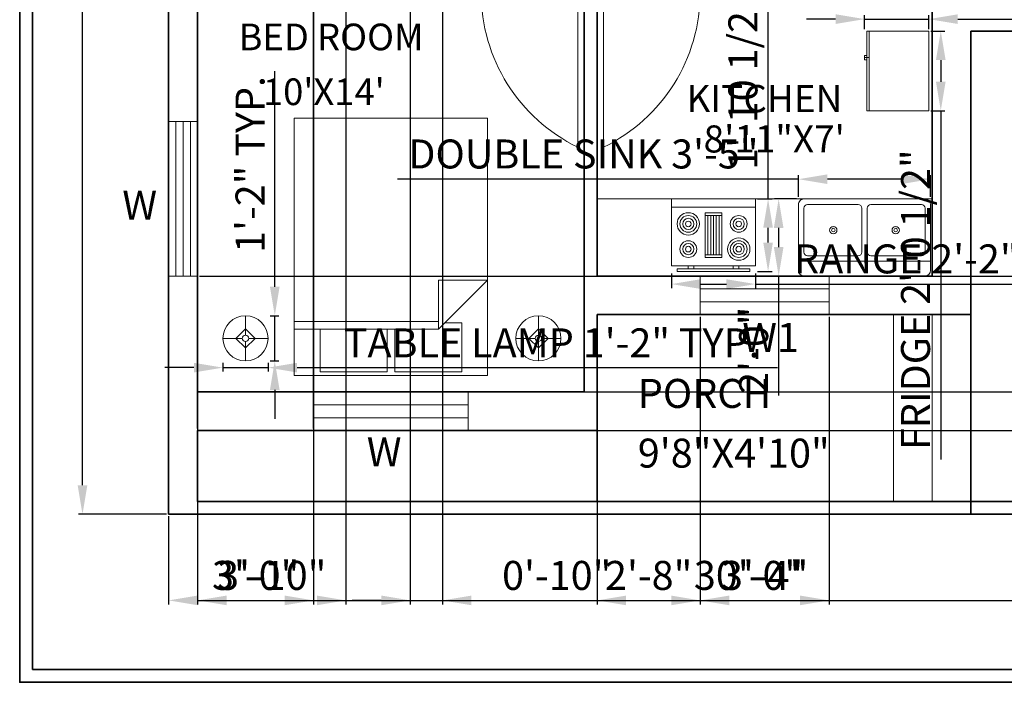
# Model space of a CAD drawing. Units: inches. Extents: x 2436 to 3928, y 1526 to 2149.
# Tile 1 of 6: x 2436 to 2742, y 1526 to 1731. Entities that reach past the tile are written whole.
import ezdxf

# ---------------------------------------------------------------- set-up
doc = ezdxf.new("R2010")
doc.units = ezdxf.units.IN
for name, color, linetype, lineweight in [('A-AREA-IDEN', 152, 'Continuous', 18), ('A-DOOR', 4, 'Continuous', 18), ('A-EQPM', 9, 'Continuous', 18), ('A-FLOR-CASE', 8, 'Continuous', 18), ('A-FLOR-FIXT', 9, 'Continuous', 18), ('A-FLOR-STRS', 7, 'Continuous', 18), ('A-FURN', 8, 'Continuous', 18), ('A-GLAZ', 2, 'Continuous', 18), ('A-GLAZ-TEXT', 114, 'Continuous', 18), ('A-WALL', 7, 'Continuous', 35), ('G-ANNO-TTLB', 7, 'Continuous', 35), ('S-ANNO-DIMS', 2, 'Continuous', 18)]:
    doc.layers.add(name, color=color, linetype=linetype, lineweight=lineweight)
doc.styles.get("Standard").update_dxf_attribs({"font": 'arial.ttf'})
doc.dimstyles.new('ISO-25', dxfattribs={"dimtxt": 9, "dimasz": 9, "dimexe": 1.25, "dimexo": 0.625, "dimgap": 2, "dimtad": 1, "dimdec": 1, "dimlunit": 4, "dimtxsty": 'Standard', "dimcen": 2.5, "dimadec": 0, "dimazin": 0, "dimtfac": 1, "dimtdec": 1, "dimtmove": 0, "dimatfit": 3, "dimfxl": 1, "dimarcsym": 0})

# ---------------------------------------------------------------- blocks, each defined once
blk = doc.blocks.new('Range-Oven - 30 in top')
for p, q in [((0, -3), (30, -3)), ((12, -6), (18, -6)), ((13, -20), (13, -6)), ((14, -6), (14, -20)), ((15, -20), (15, -6)), ((16, -6), (16, -20)), ((17, -20), (17, -6)), ((18, -20), (12, -20)), ((6, -24), (6, -25)), ((8, -25), (8, -24)), ((22, -25), (22, -24)), ((24, -24), (24, -25))]:
    blk.add_line(p, q)
for points in [[(0, -24), (0, 0), (30, 0), (30, -24)], [(12, -21), (12, -5), (18, -5), (18, -21)], [(2, -26), (2, -25), (28, -25), (28, -26)]]:
    blk.add_lwpolyline(points, close=True)
for centre, radius in [((6, -9), 4), ((6, -9), 3), ((6, -9), 2), ((24, -9), 3), ((24, -9), 2), ((6, -9), 1), ((24, -9), 1), ((24, -18), 4), ((6, -18), 3), ((6, -18), 2), ((6, -18), 1), ((24, -18), 3), ((24, -18), 2), ((24, -18), 1)]:
    blk.add_circle(centre, radius)
blk = doc.blocks.new('Sink-double - 36 in top')
for p, q in [((-18, -4), (18, -4)), ((-0.75, -18.5), (-0.75, -6.5)), ((0.75, -6.5), (0.75, -18.5))]:
    blk.add_line(p, q)
for points in [[(-16.5, 0), (16.5, 0)], [(-18, -19.5), (-18, -1.5)], [(18, -1.5), (18, -19.5)], [(-16.5, -18.5), (-16.5, -6.5)], [(-15.5, -5.5), (-1.75, -5.5)], [(1.75, -5.5), (15.5, -5.5)], [(16.5, -6.5), (16.5, -18.5)], [(16.5, -21), (-16.5, -21)], [(-1.75, -19.5), (-15.5, -19.5)], [(15.5, -19.5), (1.75, -19.5)]]:
    blk.add_lwpolyline(points)
for centre, radius in [((-8.5, -12.5), 1), ((-8.5, -12.5), 0.5), ((8.5, -12.5), 1), ((8.5, -12.5), 0.5)]:
    blk.add_circle(centre, radius)
for centre, radius, start, end in [((-16.5, -1.5), 1.5, 90, 180), ((16.5, -1.5), 1.5, 0, 90), ((-15.5, -6.5), 1, 90, 180), ((-1.75, -6.5), 1, 0, 90), ((1.75, -6.5), 1, 90, 180), ((15.5, -6.5), 1, 0, 90), ((-15.5, -18.5), 1, 180, 270), ((-1.75, -18.5), 1, 270, 0), ((1.75, -18.5), 1, 180, 270), ((15.5, -18.5), 1, 270, 0), ((-16.5, -19.5), 1.5, 180, 270), ((16.5, -19.5), 1.5, 270, 0)]:
    blk.add_arc(centre, radius, start, end)
blk = doc.blocks.new('Refrigerator-2 door - 36 in top')
for p, q in [((0, -26.999999), (36, -26.999999)), ((11, -27.999999), (11, -28.999999)), ((11, -28.999999), (13, -28.999999)), ((12, -26.999999), (12, -28.999999)), ((13, -28.999999), (13, -27.999999))]:
    blk.add_line(p, q)
blk.add_lwpolyline([(0, -27.999999), (0, 0), (36, 0), (36, -27.999999)], close=True)
blk = doc.blocks.new('Bed - Queen')
for p, q in [((0, -80.00003), (0, 0)), ((0, 0), (59.99999, 0)), ((59.99999, 0), (59.99999, -80.00003)), ((7.99999, -1.2), (28.79998, -1.2)), ((7.99999, -14.4), (7.99999, -1.2)), ((28.79998, -1.2), (28.79998, -14.4)), ((31.19999, -1.2), (51.99999, -1.2)), ((31.19999, -14.4), (31.19999, -1.2)), ((51.99999, -1.2), (51.99999, -16.4)), ((0, -14.4), (44.8, -14.4)), ((59.99999, -29.6), (44.8, -14.4)), ((44.8, -14.4), (44.8, -29.6)), ((44.8, -16.8), (0, -16.8)), ((51.99999, -16.4), (46.79936, -16.4)), ((44.8, -29.6), (59.99999, -29.6)), ((59.99999, -80.00003), (0, -80.00003))]:
    blk.add_line(p, q)
blk = doc.blocks.new('Lamp - Table')
for p, q in [((0, 7), (0, 1)), ((-1, 0), (-7, 0)), ((0, 3), (-3, 0)), ((-3, 0), (0, -3)), ((3, 0), (0, 3)), ((0, -3), (3, 0)), ((1, 0), (7, 0)), ((0, -1), (0, -7))]:
    blk.add_line(p, q)
for radius in [7, 1]:
    blk.add_circle((0, 0), radius)
blk = doc.blocks.new('WIN-48x9-PLAN')
for p, q in [((0, 0), (0, 9)), ((0, 6.75), (48, 6.75)), ((48, 0), (48, 9)), ((0, 4.5), (48, 4.5)), ((0, 2.25), (48, 2.25))]:
    blk.add_line(p, q)
blk = doc.blocks.new('DOOR-SINGLE-30-PLAN')
blk.add_line((0, 0), (0, 48))
blk.add_arc((-23.4, 0), 53.4, 0, 64.0108)
blk = doc.blocks.new('*D32')
at = {"layer": 'Defpoints', "color": 0, "transparency": 16777216}
for p in [(2499.08, 1625.43), (2513.08, 1625.43), (2513.08, 1623.33)]:
    blk.add_point(p, dxfattribs=at)
at = {"layer": 'S-ANNO-DIMS', "color": 0, "lineweight": -2, "transparency": 16777216}
for p, q in [((2490.08, 1623.33), (2481.08, 1623.33)), ((2499.08, 1624.8), (2499.08, 1622.08)), ((2499.08, 1623.33), (2513.08, 1623.33)), ((2513.08, 1624.8), (2513.08, 1622.08)), ((2522.08, 1623.33), (2671.22, 1623.33))]:
    blk.add_line(p, q, dxfattribs=at)
at = {"layer": 'S-ANNO-DIMS', "color": 0, "transparency": 16777216}
for points in [[(2490.08, 1624.83), (2490.08, 1621.83), (2499.08, 1623.33)], [(2522.08, 1624.83), (2522.08, 1621.83), (2513.08, 1623.33)]]:
    blk.add_solid(points, dxfattribs=at)
at = {"layer": 'S-ANNO-DIMS', "color": 0, "transparency": 16777216, "insert": (2601.15, 1629.85), "char_height": 9, "attachment_point": 5}
blk.add_mtext('TABLE LAMP 1\'-2" TYP.', dxfattribs=at)
blk = doc.blocks.new('*D33')
at = {"layer": 'Defpoints', "color": 0, "transparency": 16777216}
for p in [(2513.08, 1639.43), (2515.18, 1639.43), (2513.08, 1625.43)]:
    blk.add_point(p, dxfattribs=at)
at = {"layer": 'S-ANNO-DIMS', "color": 0, "lineweight": -2, "transparency": 16777216}
for p, q in [((2515.18, 1648.43), (2515.18, 1715.44)), ((2513.7, 1639.43), (2516.43, 1639.43)), ((2515.18, 1625.43), (2515.18, 1639.43)), ((2513.7, 1625.43), (2516.43, 1625.43)), ((2515.18, 1616.43), (2515.18, 1607.43))]:
    blk.add_line(p, q, dxfattribs=at)
at = {"layer": 'S-ANNO-DIMS', "color": 0, "transparency": 16777216}
for points in [[(2513.68, 1648.43), (2516.68, 1648.43), (2515.18, 1639.43)], [(2513.68, 1616.43), (2516.68, 1616.43), (2515.18, 1625.43)]]:
    blk.add_solid(points, dxfattribs=at)
at = {"layer": 'S-ANNO-DIMS', "color": 0, "transparency": 16777216, "insert": (2508.66, 1686.43), "char_height": 9, "attachment_point": 5, "rotation": 90}
blk.add_mtext('1\'-2" TYP.', dxfattribs=at)
blk = doc.blocks.new('*D50')
at = {"layer": 'Defpoints', "color": 0, "transparency": 16777216}
for p in [(2638.33, 1653.19), (2664.4, 1653.19), (2664.4, 1649.28)]:
    blk.add_point(p, dxfattribs=at)
at = {"layer": 'S-ANNO-DIMS', "color": 0, "lineweight": -2, "transparency": 16777216}
for p, q in [((2638.33, 1652.56), (2638.33, 1648.03)), ((2664.4, 1652.56), (2664.4, 1648.03)), ((2647.33, 1649.28), (2655.4, 1649.28)), ((2664.4, 1649.28), (2749.06, 1649.28))]:
    blk.add_line(p, q, dxfattribs=at)
at = {"layer": 'S-ANNO-DIMS', "color": 0, "transparency": 16777216}
for points in [[(2647.33, 1650.78), (2647.33, 1647.78), (2638.33, 1649.28)], [(2655.4, 1650.78), (2655.4, 1647.78), (2664.4, 1649.28)]]:
    blk.add_solid(points, dxfattribs=at)
at = {"layer": 'S-ANNO-DIMS', "color": 0, "transparency": 16777216, "insert": (2711.23, 1655.93), "char_height": 9, "attachment_point": 5}
blk.add_mtext('RANGE 2\'-2"', dxfattribs=at)
blk = doc.blocks.new('*D51')
at = {"layer": 'Defpoints', "color": 0, "transparency": 16777216}
for p in [(2664.4, 1675.79), (2668.31, 1675.79), (2664.4, 1653.19)]:
    blk.add_point(p, dxfattribs=at)
at = {"layer": 'S-ANNO-DIMS', "color": 0, "lineweight": -2, "transparency": 16777216}
for p, q in [((2668.31, 1675.79), (2668.31, 1739.83)), ((2665.03, 1675.79), (2669.56, 1675.79)), ((2668.31, 1662.19), (2668.31, 1666.79)), ((2665.03, 1653.19), (2669.56, 1653.19))]:
    blk.add_line(p, q, dxfattribs=at)
at = {"layer": 'S-ANNO-DIMS', "color": 0, "transparency": 16777216}
for points in [[(2666.81, 1666.79), (2669.81, 1666.79), (2668.31, 1675.79)], [(2666.81, 1662.19), (2669.81, 1662.19), (2668.31, 1653.19)]]:
    blk.add_solid(points, dxfattribs=at)
at = {"layer": 'S-ANNO-DIMS', "color": 0, "transparency": 16777216, "insert": (2661.66, 1712.31), "char_height": 9, "attachment_point": 5, "rotation": 90}
blk.add_mtext('1\'-10 1/2"', dxfattribs=at)
blk = doc.blocks.new('*D52')
at = {"layer": 'Defpoints', "color": 0, "transparency": 16777216}
for p in [(2677.74, 1681.86), (2677.74, 1675.71), (2718.75, 1675.71)]:
    blk.add_point(p, dxfattribs=at)
at = {"layer": 'S-ANNO-DIMS', "color": 0, "lineweight": -2, "transparency": 16777216}
for p, q in [((2677.74, 1681.86), (2553.23, 1681.86)), ((2677.74, 1676.34), (2677.74, 1683.11)), ((2709.75, 1681.86), (2686.74, 1681.86)), ((2718.75, 1676.34), (2718.75, 1683.11))]:
    blk.add_line(p, q, dxfattribs=at)
at = {"layer": 'S-ANNO-DIMS', "color": 0, "transparency": 16777216}
for points in [[(2686.74, 1683.36), (2686.74, 1680.36), (2677.74, 1681.86)], [(2709.75, 1683.36), (2709.75, 1680.36), (2718.75, 1681.86)]]:
    blk.add_solid(points, dxfattribs=at)
at = {"layer": 'S-ANNO-DIMS', "color": 0, "transparency": 16777216, "insert": (2610.98, 1688.52), "char_height": 9, "attachment_point": 5}
blk.add_mtext('DOUBLE SINK 3\'-5"', dxfattribs=at)
blk = doc.blocks.new('*D53')
at = {"layer": 'Defpoints', "color": 0, "transparency": 16777216}
for p in [(2677.74, 1675.71), (2671.59, 1651.79), (2677.74, 1651.79)]:
    blk.add_point(p, dxfattribs=at)
at = {"layer": 'S-ANNO-DIMS', "color": 0, "lineweight": -2, "transparency": 16777216}
for p, q in [((2677.11, 1675.71), (2670.34, 1675.71)), ((2671.59, 1666.71), (2671.59, 1660.79)), ((2677.11, 1651.79), (2670.34, 1651.79)), ((2671.59, 1651.79), (2671.59, 1614.71))]:
    blk.add_line(p, q, dxfattribs=at)
at = {"layer": 'S-ANNO-DIMS', "color": 0, "transparency": 16777216}
for points in [[(2670.09, 1666.71), (2673.09, 1666.71), (2671.59, 1675.71)], [(2670.09, 1660.79), (2673.09, 1660.79), (2671.59, 1651.79)]]:
    blk.add_solid(points, dxfattribs=at)
at = {"layer": 'S-ANNO-DIMS', "color": 0, "transparency": 16777216, "insert": (2664.99, 1628.75), "char_height": 9, "attachment_point": 5, "rotation": 90}
blk.add_mtext('2\'-0"', dxfattribs=at)
blk = doc.blocks.new('*D54')
at = {"layer": 'Defpoints', "color": 0, "transparency": 16777216}
for p in [(2718.2, 1727.86), (2718.2, 1703.12), (2721.91, 1703.12)]:
    blk.add_point(p, dxfattribs=at)
at = {"layer": 'S-ANNO-DIMS', "color": 0, "lineweight": -2, "transparency": 16777216}
for p, q in [((2718.82, 1727.86), (2723.16, 1727.86)), ((2721.91, 1718.86), (2721.91, 1712.12)), ((2718.82, 1703.12), (2723.16, 1703.12)), ((2721.91, 1703.12), (2721.91, 1594.75))]:
    blk.add_line(p, q, dxfattribs=at)
at = {"layer": 'S-ANNO-DIMS', "color": 0, "transparency": 16777216}
for points in [[(2720.41, 1718.86), (2723.41, 1718.86), (2721.91, 1727.86)], [(2720.41, 1712.12), (2723.41, 1712.12), (2721.91, 1703.12)]]:
    blk.add_solid(points, dxfattribs=at)
at = {"layer": 'S-ANNO-DIMS', "color": 0, "transparency": 16777216, "insert": (2715.25, 1644.44), "char_height": 9, "attachment_point": 5, "rotation": 90}
blk.add_mtext('FRIDGE 2\'-0 1/2"', dxfattribs=at)
blk = doc.blocks.new('*D55')
at = {"layer": 'Defpoints', "color": 0, "transparency": 16777216}
for p in [(2718.2, 1731.57), (2698.27, 1727.86), (2718.2, 1727.86)]:
    blk.add_point(p, dxfattribs=at)
at = {"layer": 'S-ANNO-DIMS', "color": 0, "lineweight": -2, "transparency": 16777216}
for p, q in [((2689.27, 1731.57), (2680.27, 1731.57)), ((2698.27, 1728.48), (2698.27, 1732.82)), ((2698.27, 1731.57), (2718.2, 1731.57)), ((2718.2, 1728.48), (2718.2, 1732.82)), ((2727.2, 1731.57), (2763.27, 1731.57))]:
    blk.add_line(p, q, dxfattribs=at)
at = {"layer": 'S-ANNO-DIMS', "color": 0, "transparency": 16777216}
for points in [[(2689.27, 1733.07), (2689.27, 1730.07), (2698.27, 1731.57)], [(2727.2, 1733.07), (2727.2, 1730.07), (2718.2, 1731.57)]]:
    blk.add_solid(points, dxfattribs=at)
at = {"layer": 'S-ANNO-DIMS', "color": 0, "transparency": 16777216, "insert": (2749.73, 1738.16), "char_height": 9, "attachment_point": 5}
blk.add_mtext('1\'-8"', dxfattribs=at)
blk = doc.blocks.new('*D56')
at = {"layer": 'Defpoints', "color": 0, "transparency": 16777216}
for p in [(2482.24, 1577.79), (2842.24, 1577.79), (2842.24, 1551.04)]:
    blk.add_point(p, dxfattribs=at)
at = {"layer": 'S-ANNO-DIMS', "color": 0, "lineweight": -2, "transparency": 16777216}
for p, q in [((2482.24, 1577.16), (2482.24, 1549.79)), ((2842.24, 1577.16), (2842.24, 1549.79)), ((2491.24, 1551.04), (2833.24, 1551.04))]:
    blk.add_line(p, q, dxfattribs=at)
at = {"layer": 'S-ANNO-DIMS', "color": 0, "transparency": 16777216}
for points in [[(2491.24, 1552.54), (2491.24, 1549.54), (2482.24, 1551.04)], [(2833.24, 1552.54), (2833.24, 1549.54), (2842.24, 1551.04)]]:
    blk.add_solid(points, dxfattribs=at)
at = {"layer": 'S-ANNO-DIMS', "color": 0, "transparency": 16777216, "insert": (2662.24, 1557.64), "char_height": 9, "attachment_point": 5}
blk.add_mtext('30\'-0"', dxfattribs=at)
blk = doc.blocks.new('*D57')
at = {"layer": 'Defpoints', "color": 0, "transparency": 16777216}
for p in [(2455.49, 2017.79), (2482.24, 2017.79), (2482.24, 1577.79)]:
    blk.add_point(p, dxfattribs=at)
at = {"layer": 'S-ANNO-DIMS', "color": 0, "lineweight": -2, "transparency": 16777216}
for p, q in [((2481.61, 2017.79), (2454.24, 2017.79)), ((2455.49, 1586.79), (2455.49, 2008.79)), ((2481.61, 1577.79), (2454.24, 1577.79))]:
    blk.add_line(p, q, dxfattribs=at)
at = {"layer": 'S-ANNO-DIMS', "color": 0, "transparency": 16777216}
for points in [[(2453.99, 2008.79), (2456.99, 2008.79), (2455.49, 2017.79)], [(2453.99, 1586.79), (2456.99, 1586.79), (2455.49, 1577.79)]]:
    blk.add_solid(points, dxfattribs=at)
at = {"layer": 'S-ANNO-DIMS', "color": 0, "transparency": 16777216, "insert": (2448.89, 1797.79), "char_height": 9, "attachment_point": 5, "rotation": 90}
blk.add_mtext('36\'-8"', dxfattribs=at)
blk = doc.blocks.new('*D58')
at = {"layer": 'Defpoints', "color": 0, "transparency": 16777216}
for p in [(2491.24, 2008.79), (2527.24, 2008.79), (2527.24, 1551.04)]:
    blk.add_point(p, dxfattribs=at)
at = {"layer": 'S-ANNO-DIMS', "color": 0, "lineweight": -2, "transparency": 16777216}
for p, q in [((2491.24, 2008.16), (2491.24, 1549.79)), ((2527.24, 2008.16), (2527.24, 1549.79)), ((2500.24, 1551.04), (2518.24, 1551.04))]:
    blk.add_line(p, q, dxfattribs=at)
at = {"layer": 'S-ANNO-DIMS', "color": 0, "transparency": 16777216}
for points in [[(2500.24, 1552.54), (2500.24, 1549.54), (2491.24, 1551.04)], [(2518.24, 1552.54), (2518.24, 1549.54), (2527.24, 1551.04)]]:
    blk.add_solid(points, dxfattribs=at)
at = {"layer": 'S-ANNO-DIMS', "color": 0, "transparency": 16777216, "insert": (2509.24, 1557.64), "char_height": 9, "attachment_point": 5}
blk.add_mtext('3\'-0"', dxfattribs=at)
blk = doc.blocks.new('*D63')
at = {"layer": 'Defpoints', "color": 0, "transparency": 16777216}
for p in [(2491.24, 1651.79), (2868.99, 1651.79), (2491.24, 1615.79)]:
    blk.add_point(p, dxfattribs=at)
at = {"layer": 'S-ANNO-DIMS', "color": 0, "lineweight": -2, "transparency": 16777216}
for p, q in [((2491.86, 1651.79), (2870.24, 1651.79)), ((2868.99, 1624.79), (2868.99, 1642.79)), ((2491.86, 1615.79), (2870.24, 1615.79))]:
    blk.add_line(p, q, dxfattribs=at)
at = {"layer": 'S-ANNO-DIMS', "color": 0, "transparency": 16777216}
for points in [[(2867.49, 1642.79), (2870.49, 1642.79), (2868.99, 1651.79)], [(2867.49, 1624.79), (2870.49, 1624.79), (2868.99, 1615.79)]]:
    blk.add_solid(points, dxfattribs=at)
at = {"layer": 'S-ANNO-DIMS', "color": 0, "transparency": 16777216, "insert": (2862.39, 1633.79), "char_height": 9, "attachment_point": 5, "rotation": 90}
blk.add_mtext('3\'-0"', dxfattribs=at)
blk = doc.blocks.new('*D64')
at = {"layer": 'Defpoints', "color": 0, "transparency": 16777216}
for p in [(2527.24, 2114.67), (2491.24, 1603.79), (2527.24, 1603.79)]:
    blk.add_point(p, dxfattribs=at)
at = {"layer": 'S-ANNO-DIMS', "color": 0, "lineweight": -2, "transparency": 16777216}
for p, q in [((2491.24, 1604.41), (2491.24, 2115.92)), ((2527.24, 1604.41), (2527.24, 2115.92)), ((2500.24, 2114.67), (2518.24, 2114.67))]:
    blk.add_line(p, q, dxfattribs=at)
at = {"layer": 'S-ANNO-DIMS', "color": 0, "transparency": 16777216}
for points in [[(2500.24, 2116.17), (2500.24, 2113.17), (2491.24, 2114.67)], [(2518.24, 2116.17), (2518.24, 2113.17), (2527.24, 2114.67)]]:
    blk.add_solid(points, dxfattribs=at)
at = {"layer": 'S-ANNO-DIMS', "color": 0, "transparency": 16777216, "insert": (2509.24, 2121.27), "char_height": 9, "attachment_point": 5}
blk.add_mtext('3\'-0"', dxfattribs=at)
blk = doc.blocks.new('*D65')
at = {"layer": 'Defpoints', "color": 0, "transparency": 16777216}
for p in [(2575.24, 1615.79), (2868.99, 1615.79), (2575.24, 1603.79)]:
    blk.add_point(p, dxfattribs=at)
at = {"layer": 'S-ANNO-DIMS', "color": 0, "lineweight": -2, "transparency": 16777216}
for p, q in [((2868.99, 1624.79), (2868.99, 1660.87)), ((2575.86, 1615.79), (2870.24, 1615.79)), ((2868.99, 1603.79), (2868.99, 1615.79)), ((2575.86, 1603.79), (2870.24, 1603.79)), ((2868.99, 1594.79), (2868.99, 1585.79))]:
    blk.add_line(p, q, dxfattribs=at)
at = {"layer": 'S-ANNO-DIMS', "color": 0, "transparency": 16777216}
for points in [[(2867.49, 1624.79), (2870.49, 1624.79), (2868.99, 1615.79)], [(2867.49, 1594.79), (2870.49, 1594.79), (2868.99, 1603.79)]]:
    blk.add_solid(points, dxfattribs=at)
at = {"layer": 'S-ANNO-DIMS', "color": 0, "transparency": 16777216, "insert": (2862.39, 1647.33), "char_height": 9, "attachment_point": 5, "rotation": 90}
blk.add_mtext('1\'-0"', dxfattribs=at)
blk = doc.blocks.new('*D66')
at = {"layer": 'Defpoints', "color": 0, "transparency": 16777216}
for p in [(2647.24, 1639.79), (2687.24, 1639.79), (2687.24, 1551.04)]:
    blk.add_point(p, dxfattribs=at)
at = {"layer": 'S-ANNO-DIMS', "color": 0, "lineweight": -2, "transparency": 16777216}
for p, q in [((2647.24, 1639.16), (2647.24, 1549.79)), ((2687.24, 1639.16), (2687.24, 1549.79)), ((2656.24, 1551.04), (2678.24, 1551.04))]:
    blk.add_line(p, q, dxfattribs=at)
at = {"layer": 'S-ANNO-DIMS', "color": 0, "transparency": 16777216}
for points in [[(2656.24, 1552.54), (2656.24, 1549.54), (2647.24, 1551.04)], [(2678.24, 1552.54), (2678.24, 1549.54), (2687.24, 1551.04)]]:
    blk.add_solid(points, dxfattribs=at)
at = {"layer": 'S-ANNO-DIMS', "color": 0, "transparency": 16777216, "insert": (2667.24, 1557.64), "char_height": 9, "attachment_point": 5}
blk.add_mtext('3\'-4"', dxfattribs=at)
blk = doc.blocks.new('*D67')
at = {"layer": 'Defpoints', "color": 0, "transparency": 16777216}
for p in [(2615.24, 1639.79), (2647.24, 1639.79), (2647.24, 1551.04)]:
    blk.add_point(p, dxfattribs=at)
at = {"layer": 'S-ANNO-DIMS', "color": 0, "lineweight": -2, "transparency": 16777216}
for p, q in [((2615.24, 1639.16), (2615.24, 1549.79)), ((2647.24, 1639.16), (2647.24, 1549.79)), ((2624.24, 1551.04), (2638.24, 1551.04))]:
    blk.add_line(p, q, dxfattribs=at)
at = {"layer": 'S-ANNO-DIMS', "color": 0, "transparency": 16777216}
for points in [[(2624.24, 1552.54), (2624.24, 1549.54), (2615.24, 1551.04)], [(2638.24, 1552.54), (2638.24, 1549.54), (2647.24, 1551.04)]]:
    blk.add_solid(points, dxfattribs=at)
at = {"layer": 'S-ANNO-DIMS', "color": 0, "transparency": 16777216, "insert": (2631.24, 1557.63), "char_height": 9, "attachment_point": 5}
blk.add_mtext('2\'-8"', dxfattribs=at)
blk = doc.blocks.new('*D72')
at = {"layer": 'Defpoints', "color": 0, "transparency": 16777216}
for p in [(2491.24, 1798.29), (2537.24, 1788.29), (2537.24, 1551.04)]:
    blk.add_point(p, dxfattribs=at)
at = {"layer": 'S-ANNO-DIMS', "color": 0, "lineweight": -2, "transparency": 16777216}
for p, q in [((2491.24, 1797.66), (2491.24, 1549.79)), ((2537.24, 1787.66), (2537.24, 1549.79)), ((2500.24, 1551.04), (2528.24, 1551.04))]:
    blk.add_line(p, q, dxfattribs=at)
at = {"layer": 'S-ANNO-DIMS', "color": 0, "transparency": 16777216}
for points in [[(2500.24, 1552.54), (2500.24, 1549.54), (2491.24, 1551.04)], [(2528.24, 1552.54), (2528.24, 1549.54), (2537.24, 1551.04)]]:
    blk.add_solid(points, dxfattribs=at)
at = {"layer": 'S-ANNO-DIMS', "color": 0, "transparency": 16777216, "insert": (2514.24, 1557.64), "char_height": 9, "attachment_point": 5}
blk.add_mtext('3\'-10"', dxfattribs=at)
blk = doc.blocks.new('*D73')
at = {"layer": 'Defpoints', "color": 0, "transparency": 16777216}
for p in [(2557.24, 1798.29), (2567.24, 1798.29), (2567.24, 1551.04)]:
    blk.add_point(p, dxfattribs=at)
at = {"layer": 'S-ANNO-DIMS', "color": 0, "lineweight": -2, "transparency": 16777216}
for p, q in [((2557.24, 1797.66), (2557.24, 1549.79)), ((2567.24, 1797.66), (2567.24, 1549.79)), ((2548.24, 1551.04), (2539.24, 1551.04)), ((2557.24, 1551.04), (2567.24, 1551.04)), ((2576.24, 1551.04), (2620.16, 1551.04))]:
    blk.add_line(p, q, dxfattribs=at)
at = {"layer": 'S-ANNO-DIMS', "color": 0, "transparency": 16777216}
for points in [[(2548.24, 1552.54), (2548.24, 1549.54), (2557.24, 1551.04)], [(2576.24, 1552.54), (2576.24, 1549.54), (2567.24, 1551.04)]]:
    blk.add_solid(points, dxfattribs=at)
at = {"layer": 'S-ANNO-DIMS', "color": 0, "transparency": 16777216, "insert": (2602.7, 1557.63), "char_height": 9, "attachment_point": 5}
blk.add_mtext('0\'-10"', dxfattribs=at)

msp = doc.modelspace()

# ---------------------------------------------------------------- linework, layer by layer
at = {"layer": 'A-FLOR-CASE'}
msp.add_line((2615.24, 1675.79), (2719.24, 1675.79), dxfattribs=at)
at = {"layer": 'A-FLOR-STRS'}
for p, q in [((2707.24, 1581.79), (2707.24, 1639.79)), ((2719.24, 1581.79), (2719.24, 1639.79))]:
    msp.add_line(p, q, dxfattribs=at)
at = {"layer": 'A-GLAZ'}
for p, q in [((2647.24, 1651.79), (2647.24, 1639.79)), ((2687.24, 1651.79), (2687.24, 1639.79)), ((2647.24, 1647.79), (2687.24, 1647.79)), ((2647.24, 1643.79), (2687.24, 1643.79)), ((2527.24, 1615.79), (2527.24, 1603.79)), ((2575.24, 1615.79), (2575.24, 1603.79)), ((2527.24, 1611.79), (2575.24, 1611.79)), ((2527.24, 1607.79), (2575.24, 1607.79))]:
    msp.add_line(p, q, dxfattribs=at)
at = {"layer": 'A-WALL'}
for p, q in [((2482.24, 1577.79), (2482.24, 2017.79)), ((2491.24, 1615.79), (2491.24, 1735.79)), ((2611.24, 1615.79), (2611.24, 1735.79)), ((2615.24, 1651.79), (2615.24, 1735.79)), ((2719.24, 1651.79), (2719.24, 1735.79)), ((2731.24, 1577.79), (2731.24, 1727.79)), ((2731.24, 1727.79), (2783.24, 1727.79)), ((2615.24, 1651.79), (2719.24, 1651.79)), ((2615.24, 1581.79), (2615.24, 1639.79)), ((2615.24, 1639.79), (2731.24, 1639.79)), ((2491.24, 1615.79), (2611.24, 1615.79)), ((2482.24, 1577.79), (2482.24, 1603.79)), ((2491.24, 1581.79), (2491.24, 1603.79)), ((2491.24, 1603.79), (2615.24, 1603.79)), ((2482.24, 1581.79), (2482.24, 1595.79)), ((2491.24, 1581.79), (2833.24, 1581.79)), ((2482.24, 1577.79), (2842.24, 1577.79))]:
    msp.add_line(p, q, dxfattribs=at)
at = {"layer": 'G-ANNO-TTLB'}
for points in [[(2436, 2138.4), (3927.51, 2138.4), (3927.51, 1525.6), (2436, 1525.6)], [(2440, 2134.4), (3923.51, 2134.4), (3923.51, 1529.6), (2440, 1529.6)]]:
    msp.add_lwpolyline(points, close=True, dxfattribs=at)

# ---------------------------------------------------------------- block references
at = {"layer": 'A-DOOR', "rotation": 180}
msp.add_blockref('DOOR-SINGLE-30-PLAN', (2609.24, 1739.79), dxfattribs=at)
at = {"layer": 'A-DOOR', "extrusion": (0, 0, -1), "zscale": -1, "rotation": 180}
msp.add_blockref('DOOR-SINGLE-30-PLAN', (-2617.24, 1739.79), dxfattribs=at)
at = {"layer": 'A-EQPM', "xscale": 0.6870046739389232, "yscale": 0.6870046739389232, "zscale": 0.6870046739389232, "rotation": 270}
msp.add_blockref('Refrigerator-2 door - 36 in top', (2718.2, 1727.86), dxfattribs=at)
at = {"layer": 'A-EQPM', "xscale": 0.8692268544197554, "yscale": 0.8692268544197554, "zscale": 0.8692268544197554}
msp.add_blockref('Range-Oven - 30 in top', (2638.33, 1675.79), dxfattribs=at)
at = {"layer": 'A-FLOR-FIXT', "xscale": 1.139099176884385, "yscale": 1.139099176884385, "zscale": 1.139099176884385, "rotation": 180}
msp.add_blockref('Sink-double - 36 in top', (2698.24, 1651.79), dxfattribs=at)
at = {"layer": 'A-FURN', "xscale": -1, "rotation": 180}
msp.add_blockref('Bed - Queen', (2521.24, 1620.85), dxfattribs=at)
at = {"layer": 'A-FURN'}
for p in [(2506.08, 1632.43), (2597.01, 1632.43)]:
    msp.add_blockref('Lamp - Table', p, dxfattribs=at)
at = {"layer": 'A-GLAZ', "rotation": 270.0000000000031}
msp.add_blockref('WIN-48x9-PLAN', (2482.24, 1699.79), dxfattribs=at)

# ---------------------------------------------------------------- texts
at = {"layer": 'A-AREA-IDEN'}
for s, height, p in [('BED ROOM', 8.272, (2503.94, 1721.9)), ("   10'X14'", 8.272, (2503.94, 1704.87)), ('KITCHEN', 8.409, (2642.97, 1702.68)), ('8\'11"X7\'', 8.409, (2648.29, 1690.16)), ('PORCH', 9, (2627.87, 1610.82)), ('9\'8"X4\'10"', 9, (2627.87, 1592.28))]:
    msp.add_text(s, height=height, dxfattribs=at).set_placement(p)
at = {"layer": 'A-GLAZ-TEXT'}
for s, p in [('W', (2467.86, 1669.25)), ('W1', (2660.3, 1628.21)), ('W', (2543.74, 1592.66))]:
    msp.add_text(s, height=9, dxfattribs=at).set_placement(p)

# ---------------------------------------------------------------- dimensions: what is measured, and where the dimension line sits
at = {"layer": 'S-ANNO-DIMS'}
for base, p1, p2, picture, middle in [((2527.24, 2114.67), (2491.24, 1603.79), (2527.24, 1603.79), '*D64', (2509.24, 2121.27)), ((2527.24, 1551.04), (2491.24, 2008.79), (2527.24, 2008.79), '*D58', (2509.24, 1557.64)), ((2537.24, 1551.04), (2491.24, 1798.29), (2537.24, 1788.29), '*D72', (2514.24, 1557.64)), ((2567.24, 1551.04), (2557.24, 1798.29), (2567.24, 1798.29), '*D73', (2602.7, 1557.63)), ((2718.2, 1731.57), (2698.27, 1727.86), (2718.2, 1727.86), '*D55', (2749.73, 1738.16)), ((2647.24, 1551.04), (2615.24, 1639.79), (2647.24, 1639.79), '*D67', (2631.24, 1557.63)), ((2687.24, 1551.04), (2647.24, 1639.79), (2687.24, 1639.79), '*D66', (2667.24, 1557.64)), ((2842.24, 1551.04), (2482.24, 1577.79), (2842.24, 1577.79), '*D56', (2662.24, 1557.64))]:
    dim = msp.add_linear_dim(base=base, p1=p1, p2=p2, dimstyle='ISO-25', override={"dimdec": 1, "dimlfac": 1, "dimrnd": 0, "dimzin": 1, "dimdsep": 46, "dimlunit": 4, "dimfrac": 2}, dxfattribs=at)
    dim.commit()
    dim.dimension.update_dxf_attribs({"geometry": picture, "text_midpoint": middle})
for base, p1, p2, angle, picture, middle in [((2455.49, 2017.79), (2482.24, 1577.79), (2482.24, 2017.79), 90, '*D57', (2448.89, 1797.79)), ((2668.31, 1675.79), (2664.4, 1653.19), (2664.4, 1675.79), 90, '*D51', (2661.66, 1712.31)), ((2671.59, 1651.79), (2677.74, 1675.71), (2677.74, 1651.79), 270, '*D53', (2664.99, 1628.75)), ((2868.99, 1615.79), (2575.24, 1603.79), (2575.24, 1615.79), 90, '*D65', (2862.39, 1647.33)), ((2868.99, 1651.79), (2491.24, 1615.79), (2491.24, 1651.79), 90, '*D63', (2862.39, 1633.79))]:
    dim = msp.add_linear_dim(base=base, p1=p1, p2=p2, angle=angle, dimstyle='ISO-25', override={"dimdec": 1, "dimlfac": 1, "dimrnd": 0, "dimzin": 1, "dimdsep": 46, "dimlunit": 4, "dimfrac": 2}, dxfattribs=at)
    dim.commit()
    dim.dimension.update_dxf_attribs({"geometry": picture, "text_midpoint": middle})
for base, p1, p2, angle, text, picture, middle in [((2721.91, 1703.12), (2718.2, 1727.86), (2718.2, 1703.12), 270, 'FRIDGE <>', '*D54', (2715.25, 1644.44)), ((2515.18, 1639.43), (2513.08, 1625.43), (2513.08, 1639.43), 90, '<> TYP.', '*D33', (2508.66, 1686.43)), ((2677.74, 1681.86), (2718.75, 1675.71), (2677.74, 1675.71), 180, 'DOUBLE SINK <>', '*D52', (2610.98, 1688.52))]:
    dim = msp.add_linear_dim(base=base, p1=p1, p2=p2, angle=angle, text=text, dimstyle='ISO-25', override={"dimdec": 1, "dimlfac": 1, "dimrnd": 0, "dimzin": 1, "dimdsep": 46, "dimlunit": 4, "dimfrac": 2}, dxfattribs=at)
    dim.commit()
    dim.dimension.update_dxf_attribs({"geometry": picture, "text_midpoint": middle})
for base, p1, p2, text, picture, middle in [((2664.4, 1649.28), (2638.33, 1653.19), (2664.4, 1653.19), 'RANGE <>', '*D50', (2711.23, 1655.93)), ((2513.08, 1623.33), (2499.08, 1625.43), (2513.08, 1625.43), 'TABLE LAMP <> TYP.', '*D32', (2601.15, 1629.85))]:
    dim = msp.add_linear_dim(base=base, p1=p1, p2=p2, text=text, dimstyle='ISO-25', override={"dimdec": 1, "dimlfac": 1, "dimrnd": 0, "dimzin": 1, "dimdsep": 46, "dimlunit": 4, "dimfrac": 2}, dxfattribs=at)
    dim.commit()
    dim.dimension.update_dxf_attribs({"geometry": picture, "text_midpoint": middle})

doc.saveas('drawing.dxf')
